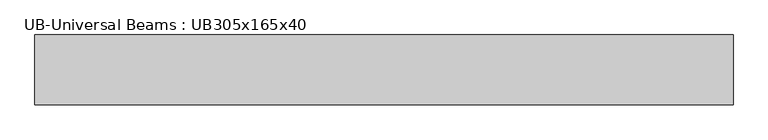
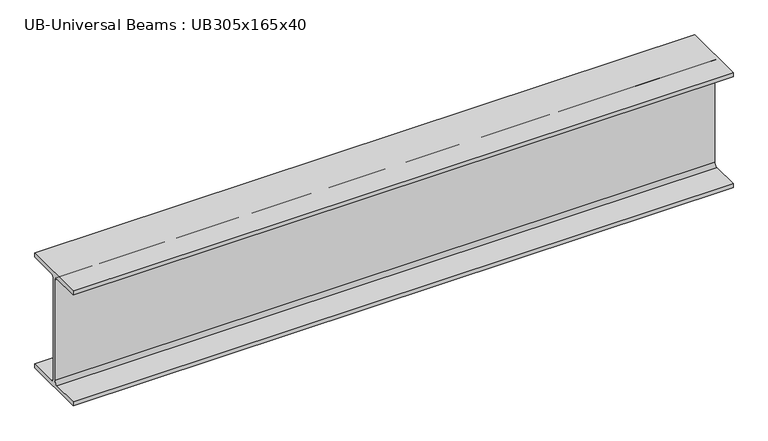
"""IFC4 building model written with IfcOpenShell, lengths in millimetres: beam geometry, UB-Universal Beams : UB305x165x40."""

from ifc_helpers import new_model, si_unit, point, frame, frame_2d, origin, place, context, project, spatial, polyline, circle_curve, trimmed, segment, composite_curve, outline, extrude, source, transform, mapped, element, save


def ub_universal_beams_ub305x165x40_f264fe8a(model_context):
    return source(origin(), model_context, "Body", "SweptSolid", [
        extrude(outline(composite_curve([segment(polyline([(82.5, -141.5), (82.5, -151.7), (-82.5, -151.7), (-82.5, -141.5), (-11.9, -141.5)]), True, "CONTINUOUS"), segment(trimmed(circle_curve(frame_2d((-11.9, -132.6)), 8.9), [point((-11.9, -141.5))], [point((-3.0, -132.6))], True, "CARTESIAN"), True, "CONTINUOUS"), segment(polyline([(-3.0, -132.6), (-3.0, 132.6)]), True, "CONTINUOUS"), segment(trimmed(circle_curve(frame_2d((-11.9, 132.6)), 8.9), [point((-3.0, 132.6))], [point((-11.9, 141.5))], True, "CARTESIAN"), True, "CONTINUOUS"), segment(polyline([(-11.9, 141.5), (-82.5, 141.5), (-82.5, 151.7), (82.5, 151.7), (82.5, 141.5), (11.9, 141.5)]), True, "CONTINUOUS"), segment(trimmed(circle_curve(frame_2d((11.9, 132.6)), 8.9), [point((11.9, 141.5))], [point((3.0, 132.6))], True, "CARTESIAN"), True, "CONTINUOUS"), segment(polyline([(3.0, 132.6), (3.0, -132.6)]), True, "CONTINUOUS"), segment(trimmed(circle_curve(frame_2d((11.9, -132.6)), 8.9), [point((3.0, -132.6))], [point((11.9, -141.5))], True, "CARTESIAN"), True, "CONTINUOUS"), segment(polyline([(11.9, -141.5), (82.5, -141.5)]), True, "CONTINUOUS")], self_intersect=False)), frame((-835.6, 0.0, 0.0), z_axis=(1.0, 0.0, 0.0), x_axis=(0.0, 1.0, 0.0)), (0.0, 0.0, 1.0), 1649.9),
    ])


if __name__ == "__main__":
    model = new_model("IFC4")
    model_context = context("Model", 3, world=origin())
    ifc_project = project(units=[si_unit("LENGTHUNIT", "METRE", prefix="MILLI")], contexts=[model_context])
    site = spatial("IfcSite", under=ifc_project)
    building = spatial("IfcBuilding", under=site)
    placement = place(None, origin())
    ub_universal_beams_ub305x165x40_shape = ub_universal_beams_ub305x165x40_f264fe8a(model_context)
    element("IfcBeam", 1, ObjectType="UB-Universal Beams : UB305x165x40", at=placement, inside=building, context=model_context, shape_type="MappedRepresentation", body=[
        mapped(ub_universal_beams_ub305x165x40_shape, transform((0.0, 0.0, 0.0), x_axis=(1.0, 0.0, 0.0), y_axis=(0.0, 1.0, 0.0), z_axis=(0.0, 0.0, 1.0))),
    ])
    save(model, "model.ifc")

# Revit data of these elements
# Type "UB-Universal Beams : UB305x165x40"
#   Section Name Key = "UB305X165X40"
#   Width = 16.5 cm
#   Web Thickness = 0.6 cm
#   Web Fillet = 0.89 cm
#   Warping Constant = 164000.0 cm⁶
#   Torsional Moment of Inertia = 14.70 cm⁴
#   Section Area = 51.3 cm²
#   Plastic Modulus weak axis = 142.0 cm³
#   Plastic Modulus strong axis = 623.0 cm³
#   Nominal Weight = 40.2999 kgf/m
#   Moment of Inertia weak axis = 764.00 cm⁴
#   Moment of Inertia strong axis = 8503.00 cm⁴
#   Height = 30.34 cm
#   Flange Thickness = 1.02 cm
#   Elastic Modulus weak axis = 92.6 cm³
#   Elastic Modulus strong axis = 560.0 cm³
#   Centroid Vertical = 15.17 cm
#   Centroid Horizontal = 8.25 cm
#   Bolt Spacing = 9.0 cm
#   Length [instance default] = 1500 mm
#   Structural Material [instance default] = Metal - Steel 43-275
#   Type Comments = ""
#   Assembly Code = ""
# Element 1 (IfcBeam, "UB-Universal Beams : UB305x165x40")
#   Materials on its faces: "Metal - Steel 43-275"
# Materials
#   "Metal - Steel 43-275": class "Metal", colour RGB 247 247 247, transparency 0, Cost = 0
